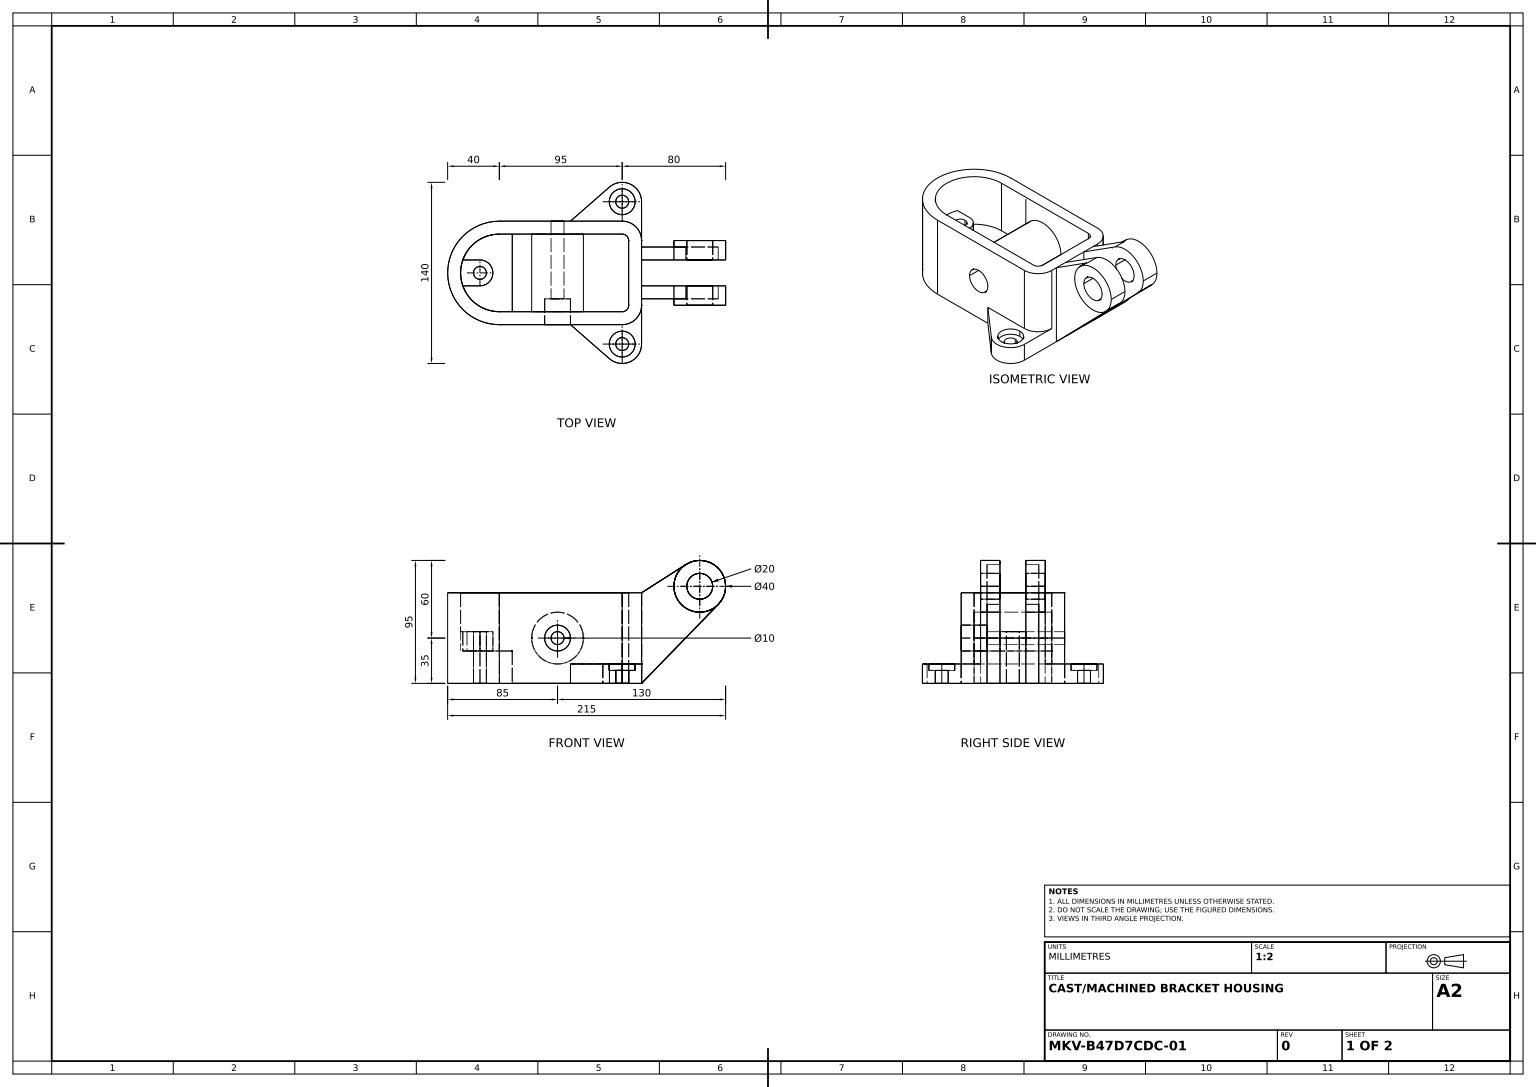
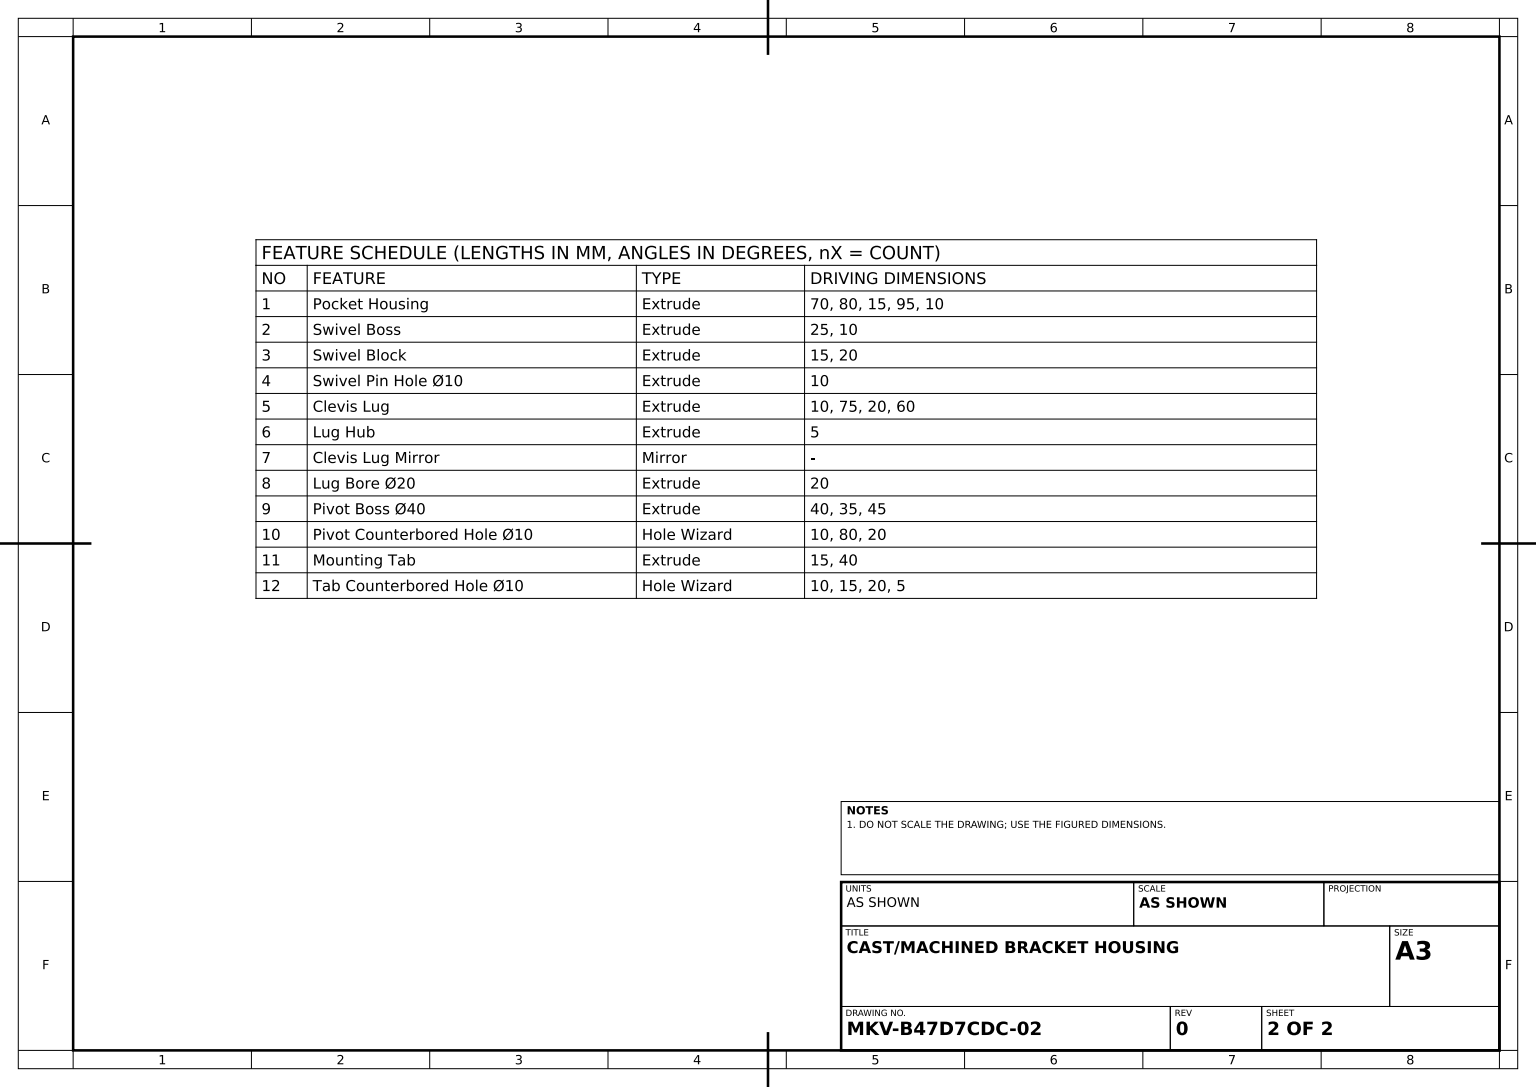
SolidWorks part; units mm, degrees
material "Plain Carbon Steel"
ref_plane "Front Plane" through (0, 0, 0) normal (0, 0, 1) x (1, 0, 0)
ref_plane "Top Plane" through (0, 0, 0) normal (0, 1, 0) x (1, 0, 0)
ref_plane "Right Plane" through (0, 0, 0) normal (1, 0, 0) x (0, 0, -1)
sketch "Pocket Housing Sketch" plane through (0, 0, 0) normal (0, 1, 0) x (1, 0, 0)
  line L0 (0, 0) -> (0, 25)
  line L1 (-15, 40) -> (-110, 40)
  line L2 (-110, -40) -> (-15, -40)
  line L3 (0, -25) -> (0, 0)
  line L4 (-15, 30) -> (-110, 30)
  line L5 (-110, -30) -> (-15, -30)
  line L6 (-10, -25) -> (-10, 0)
  line L7 (-10, 0) -> (-10, 25)
  arc A0 (-110, 40) -> (-110, -40) centre (-110, 0) ccw
  arc A1 (-15, -40) -> (0, -25) centre (-15, -25) ccw
  arc A2 (0, 25) -> (-15, 40) centre (-15, 25) ccw
  arc A3 (-110, 30) -> (-110, -30) centre (-110, 0) ccw
  arc A4 (-15, -30) -> (-10, -25) centre (-15, -25) ccw
  arc A5 (-10, 25) -> (-15, 30) centre (-15, 25) ccw
  dimension "D2" = 15
  dimension "D1" = 80
  dimension "D3" = 95
  dimension "D4" = 10
extrude "Pocket Housing" add sketch "Pocket Housing Sketch" along normal blind 70
sketch "Swivel Boss Sketch" plane through (0, 0, 0) normal (0, 1, 0) x (1, 0, 0)
  line L0 (-100, 30) -> (-100, -30)
  line L1 (-15, 30) -> (-110, 30) construction
  line L2 (-110, -30) -> (-15, -30) construction
  line L3 (-110, -30) -> (-100, -30)
  line L4 (-100, 30) -> (-110, 30)
  arc A0 (-110, 30) -> (-110, -30) centre (-110, 0) ccw construction
  arc A1 (-110, 30) -> (-110, -30) centre (-110, 0) ccw
  dimension "D1" = 10
extrude "Swivel Boss" add sketch "Swivel Boss Sketch" along normal blind 25
sketch "Swivel Block Sketch" plane through (0, 25, 0) normal (0, 1, 0) x (1, 0, 0)
  line L0 (-125, -10) -> (-138.2843, -10)
  line L1 (-125, 10) -> (-138.2843, 10)
  arc A0 (-125, -10) -> (-125, 10) centre (-125, 0) ccw
  arc A1 (-110, 30) -> (-110, -30) centre (-110, 0) ccw construction
  arc A2 (-110, 30) -> (-110, -30) centre (-110, 0) ccw construction
  arc A3 (-138.2843, 10) -> (-138.2843, -10) centre (-110, 0) ccw
  dimension "D1" = 20
  dimension "D2" = 15
extrude "Swivel Block" add sketch "Swivel Block Sketch" along normal blind 15
sketch "Swivel Pin Hole Sketch" plane through (0, 40, 0) normal (0, 1, 0) x (1, 0, 0)
  circle A0 centre (-125, 0) radius 5
  arc A1 (-125, -10) -> (-125, 10) centre (-125, 0) ccw construction
  dimension "D1" = 10
extrude "Swivel Pin Hole Ø10" cut sketch "Swivel Pin Hole Sketch" against normal through all
sketch "Clevis Lug Sketch" plane through (0, 0, 0) normal (0, 0, 1) x (1, 0, 0)
  line L0 (0, 70) -> (34.238, 91.8576)
  line L1 (0, 70) -> (0, 0)
  line L2 (0, 0) -> (59.3425, 61.0611)
  line L3 (-15, 70) -> (-15, 0) construction
  arc A0 (59.3425, 61.0611) -> (34.238, 91.8576) centre (45, 75) ccw
  dimension "D2" = 20
  dimension "D1" = 75
  dimension "D3" = 60
extrude "Clevis Lug" add sketch "Clevis Lug Sketch" along normal blind 10 from offset 10
sketch "Lug Hub Sketch" plane through (0, 0, 20) normal (0, 0, 1) x (1, 0, 0)
  circle A0 centre (45, 75) radius 20
  arc A1 (59.3425, 61.0611) -> (34.238, 91.8576) centre (45, 75) ccw construction
extrude "Lug Hub" add sketch "Lug Hub Sketch" along normal blind 5
mirror "Clevis Lug Mirror" about plane through (0, 0, 0) normal (0, 0, 1) of "Clevis Lug", "Lug Hub"
sketch "Lug Bore Sketch" plane through (0, 0, 25) normal (0, 0, 1) x (1, 0, 0)
  circle A0 centre (45, 75) radius 10
  circle A1 centre (45, 75) radius 20 construction
  dimension "D1" = 20
extrude "Lug Bore Ø20" cut sketch "Lug Bore Sketch" against normal through all and the other way through all
sketch "Pivot Boss Sketch" plane through (0, 0, 40) normal (0, 0, 1) x (1, 0, 0)
  line L0 (-110, 70) -> (-110, 0) construction
  circle A0 centre (-65, 35) radius 20
  dimension "D1" = 40
  dimension "D2" = 35
  dimension "D3" = 45
extrude "Pivot Boss Ø40" add sketch "Pivot Boss Sketch" against normal up to surface (80 mm away) up to face at (-62.5, 35, -40)
hole_wizard "Pivot Counterbored Hole Ø10" positions "3DSketch1" profile "Sketch11" legacy end condition up to next
sketch3d "3DSketch1"
  circle A0 centre (-65, 35, 30) radius 20 construction
  point P0 (-65, 35, 40)
  point P5 (-65, 35, 10)
  point P6 (-65, 35, 40)
sketch "Sketch11" plane through (-65, 35, 40) normal (1, 0, 0) x (0, -1, 0)
  line L0 (0, 0) -> (0, 80)
  line L1 (0, 80) -> (5, 80)
  line L2 (5, 80) -> (5, 20)
  line L3 (5, 20) -> (10, 20)
  line L4 (10, 20) -> (10, 0)
  line L5 (10, 0) -> (0, 0)
  line L6 (0, 110) -> (0, -10) construction
  dimension "Diameter" = 10
  dimension "Depth" = 80
  dimension "C-Bore Diameter" = 20
  dimension "C-Bore Depth" = 20
sketch "Mounting Tab Sketch" plane through (0, 0, 0) normal (0, 1, 0) x (1, 0, 0)
  line L0 (0, 25) -> (0, 55)
  line L1 (-15, 40) -> (-110, 40) construction
  line L2 (-24.863, 66.3014) -> (-55, 40)
  line L3 (-15, 40) -> (-55, 40)
  line L4 (0, 0) -> (77.1029, 0) construction
  line L5 (0, -25) -> (0, -55)
  line L6 (-15, -40) -> (-55, -40)
  line L7 (-24.863, -66.3014) -> (-55, -40)
  arc A0 (0, 55) -> (-24.863, 66.3014) centre (-15, 55) ccw
  arc A1 (0, 25) -> (-15, 40) centre (-15, 25) ccw construction
  arc A2 (0, 25) -> (-15, 40) centre (-15, 25) ccw
  arc A3 (0, -55) -> (-24.863, -66.3014) centre (-15, -55) cw
  arc A4 (0, -25) -> (-15, -40) centre (-15, -25) cw
  dimension "D2" = 15
  dimension "D1" = 15
  dimension "D3" = 40
extrude "Mounting Tab" add sketch "Mounting Tab Sketch" along normal blind 15
hole_wizard "Tab Counterbored Hole Ø10" positions "3DSketch2" profile "Sketch13" legacy end condition up to next
sketch3d "3DSketch2"
  arc A0 (-24.863, 15, 66.3014) -> (0, 15, 55) centre (-15, 15, 55) ccw construction
  arc A1 (0, 15, -55) -> (-24.863, 15, -66.3014) centre (-15, 15, -55) ccw construction
  point P0 (-15, 15, 55)
  point P2 (-15, 15, -55)
  point P8 (-15, 30, 55)
  point P12 (-15, 30, -55)
sketch "Sketch13" plane through (-15, 15, 55) normal (1, 0, 0) x (0, 0, 1)
  line L0 (0, 0) -> (0, 15)
  line L1 (0, 15) -> (5, 15)
  line L2 (5, 15) -> (5, 5)
  line L3 (5, 5) -> (10, 5)
  line L4 (10, 5) -> (10, 0)
  line L5 (10, 0) -> (0, 0)
  line L6 (0, 110) -> (0, -10) construction
  dimension "Diameter" = 10
  dimension "Depth" = 15
  dimension "C-Bore Diameter" = 20
  dimension "C-Bore Depth" = 5
